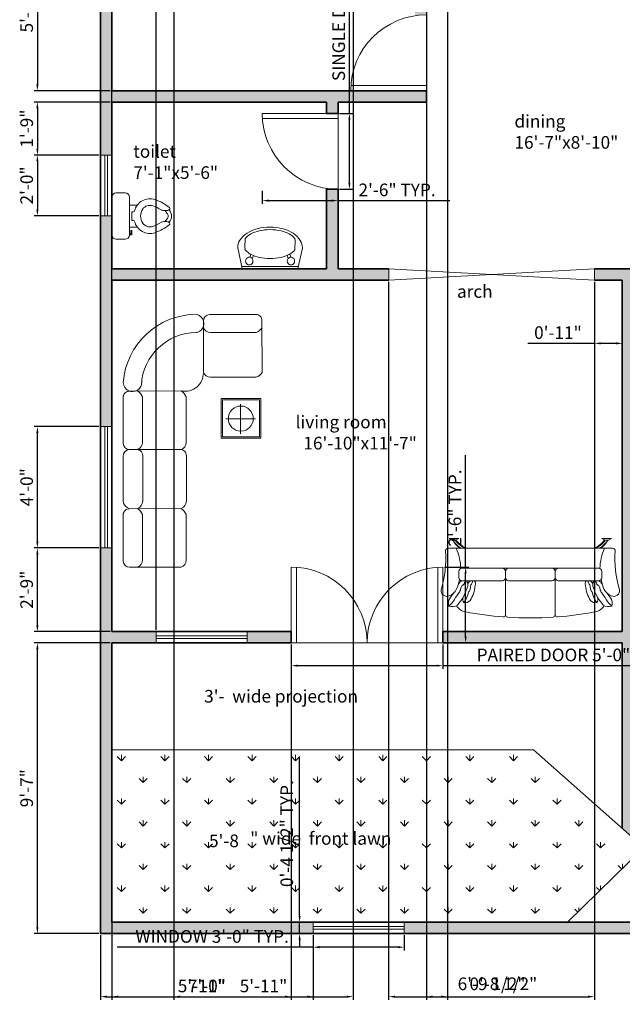
# Model space of a CAD drawing. Units: inches. Extents: x 2576 to 2974, y 2059 to 2656.
# Tile 1 of 4: x 2581 to 2819, y 2059 to 2448. Entities that reach past the tile are written whole.
import ezdxf

# ---------------------------------------------------------------- set-up
doc = ezdxf.new("R2010")
doc.units = ezdxf.units.IN
for name, color, linetype, lineweight in [('A-ANNO-DIMS', 101, 'Continuous', 18), ('A-ANNO-TEXT', 101, 'Continuous', 18), ('A-AREA-IDEN', 101, 'Continuous', 18), ('A-FLOR-FIXT', 195, 'Continuous', 18), ('A-WALL-PATT', 233, 'Continuous', 13), ('doors', 235, 'Continuous', 18), ('Furniture', 195, 'Continuous', 15), ('L-PLNT', 143, 'Continuous', 18), ('L-PLNT-PATT', 85, 'Continuous', 13), ('wall', 143, 'Continuous', 35), ('windows', 85, 'Continuous', 18)]:
    doc.layers.add(name, color=color, linetype=linetype, lineweight=lineweight)
doc.styles.get("Standard").update_dxf_attribs({"font": 'txt', "height": 5})
doc.dimstyles.new('ISO-25', dxfattribs={"dimtxt": 5, "dimasz": 2.5, "dimexe": 1.25, "dimexo": 0.625, "dimtad": 1, "dimlunit": 3, "dimtxsty": 'Standard', "dimcen": 2.5, "dimadec": 0, "dimazin": 0, "dimtfac": 1, "dimtmove": 0, "dimatfit": 3, "dimfxl": 1, "dimarcsym": 0})

# ---------------------------------------------------------------- blocks, each defined once
blk = doc.blocks.new('DOOR-SWING-30IN')
for p, q in [((0, 30), (30, 30)), ((0.07, 28), (30, 28)), ((30, 30), (30, 0))]:
    blk.add_line(p, q)
blk.add_arc((30, 30), 30, 180, 270)
blk = doc.blocks.new('DOOR-PAIR-60IN')
for p, q in [((0, 30), (0, 0)), ((2, 29.93), (2, 0)), ((58, 29.93), (58, 0)), ((60, 30), (60, 0)), ((0, 0), (30, 0)), ((60, 0), (30, 0))]:
    blk.add_line(p, q)
for centre, start, end in [((0, 0), 0, 90), ((60, 0), 90, 180)]:
    blk.add_arc(centre, 30, start, end)
blk = doc.blocks.new('WINDOW-36IN')
for p, q in [((0, 36), (0, 0)), ((4.5, 36), (0, 36)), ((1.75, 36), (1.75, 0)), ((2.75, 36), (2.75, 0)), ((4.5, 0), (4.5, 36)), ((0, 0), (4.5, 0))]:
    blk.add_line(p, q)
blk = doc.blocks.new('*D9')
at = {"layer": 'A-ANNO-DIMS', "color": 0, "lineweight": -2, "transparency": 16777216}
for p, q in [((2696.75, 2086.25), (2696.75, 2080.23)), ((2732.75, 2086.25), (2732.75, 2080.23)), ((2696.75, 2081.48), (2619.2, 2081.48)), ((2730.25, 2081.48), (2699.25, 2081.48))]:
    blk.add_line(p, q, dxfattribs=at)
at = {"layer": 'A-ANNO-DIMS', "color": 0, "transparency": 16777216}
for points in [[(2699.25, 2081.89), (2699.25, 2081.06), (2696.75, 2081.48)], [(2730.25, 2081.89), (2730.25, 2081.06), (2732.75, 2081.48)]]:
    blk.add_solid(points, dxfattribs=at)
at = {"layer": 'Defpoints', "color": 0, "transparency": 16777216}
for p in [(2696.75, 2086.88), (2732.75, 2086.88), (2696.75, 2081.48)]:
    blk.add_point(p, dxfattribs=at)
at = {"layer": 'A-ANNO-DIMS', "color": 0, "transparency": 16777216, "insert": (2656.73, 2085.08), "char_height": 5, "attachment_point": 5}
blk.add_mtext('WINDOW 3\'-0" TYP.', dxfattribs=at)
blk = doc.blocks.new('*D10')
at = {"layer": 'A-ANNO-DIMS', "color": 0, "lineweight": -2, "transparency": 16777216}
for p, q in [((2691.35, 2093.88), (2691.35, 2156.44)), ((2696.13, 2091.38), (2690.1, 2091.38)), ((2691.35, 2086.88), (2691.35, 2091.38)), ((2696.13, 2086.88), (2690.1, 2086.88)), ((2691.35, 2084.38), (2691.35, 2081.88))]:
    blk.add_line(p, q, dxfattribs=at)
at = {"layer": 'A-ANNO-DIMS', "color": 0, "transparency": 16777216}
for points in [[(2690.94, 2093.88), (2691.77, 2093.88), (2691.35, 2091.38)], [(2690.94, 2084.38), (2691.77, 2084.38), (2691.35, 2086.88)]]:
    blk.add_solid(points, dxfattribs=at)
at = {"layer": 'Defpoints', "color": 0, "transparency": 16777216}
for p in [(2691.35, 2091.38), (2696.75, 2091.38), (2696.75, 2086.88)]:
    blk.add_point(p, dxfattribs=at)
at = {"layer": 'A-ANNO-DIMS', "color": 0, "transparency": 16777216, "insert": (2686.92, 2126.41), "char_height": 5, "attachment_point": 5, "rotation": 90}
blk.add_mtext('0\'-4 1/2" TYP.', dxfattribs=at)
blk = doc.blocks.new('*D11')
at = {"layer": 'A-ANNO-DIMS', "color": 0, "lineweight": -2, "transparency": 16777216}
for p, q in [((2688.06, 2201.25), (2688.06, 2191.63)), ((2748.06, 2201.25), (2748.06, 2191.63)), ((2690.56, 2192.88), (2745.56, 2192.88)), ((2748.06, 2192.88), (2848.47, 2192.88))]:
    blk.add_line(p, q, dxfattribs=at)
at = {"layer": 'A-ANNO-DIMS', "color": 0, "transparency": 16777216}
for points in [[(2690.56, 2193.29), (2690.56, 2192.46), (2688.06, 2192.88)], [(2745.56, 2193.29), (2745.56, 2192.46), (2748.06, 2192.88)]]:
    blk.add_solid(points, dxfattribs=at)
at = {"layer": 'Defpoints', "color": 0, "transparency": 16777216}
for p in [(2688.06, 2201.88), (2748.06, 2201.88), (2748.06, 2192.88)]:
    blk.add_point(p, dxfattribs=at)
at = {"layer": 'A-ANNO-DIMS', "color": 0, "transparency": 16777216, "insert": (2799.51, 2196.48), "char_height": 5, "attachment_point": 5}
blk.add_mtext('PAIRED DOOR 5\'-0" TYP.', dxfattribs=at)
blk = doc.blocks.new('*D12')
at = {"layer": 'A-ANNO-DIMS', "color": 0, "lineweight": -2, "transparency": 16777216}
for p, q in [((2757.06, 2231.88), (2757.06, 2276.1)), ((2748.68, 2231.88), (2758.31, 2231.88)), ((2757.06, 2204.38), (2757.06, 2229.38)), ((2748.68, 2201.88), (2758.31, 2201.88))]:
    blk.add_line(p, q, dxfattribs=at)
at = {"layer": 'A-ANNO-DIMS', "color": 0, "transparency": 16777216}
for points in [[(2756.64, 2229.38), (2757.47, 2229.38), (2757.06, 2231.88)], [(2756.64, 2204.38), (2757.47, 2204.38), (2757.06, 2201.88)]]:
    blk.add_solid(points, dxfattribs=at)
at = {"layer": 'Defpoints', "color": 0, "transparency": 16777216}
for p in [(2748.06, 2231.88), (2757.06, 2231.88), (2748.06, 2201.88)]:
    blk.add_point(p, dxfattribs=at)
at = {"layer": 'A-ANNO-DIMS', "color": 0, "transparency": 16777216, "insert": (2753.46, 2255.24), "char_height": 5, "attachment_point": 5, "rotation": 90}
blk.add_mtext('2\'-6" TYP.', dxfattribs=at)
blk = doc.blocks.new('*D13')
at = {"layer": 'A-ANNO-DIMS', "color": 0, "lineweight": -2, "transparency": 16777216}
for p, q in [((2711.06, 2411.38), (2711.06, 2510.6)), ((2707.18, 2411.38), (2712.31, 2411.38)), ((2711.06, 2383.88), (2711.06, 2408.88)), ((2707.18, 2381.38), (2712.31, 2381.38))]:
    blk.add_line(p, q, dxfattribs=at)
at = {"layer": 'A-ANNO-DIMS', "color": 0, "transparency": 16777216}
for points in [[(2710.64, 2408.88), (2711.47, 2408.88), (2711.06, 2411.38)], [(2710.64, 2383.88), (2711.47, 2383.88), (2711.06, 2381.38)]]:
    blk.add_solid(points, dxfattribs=at)
at = {"layer": 'Defpoints', "color": 0, "transparency": 16777216}
for p in [(2706.56, 2411.38), (2711.06, 2411.38), (2706.56, 2381.38)]:
    blk.add_point(p, dxfattribs=at)
at = {"layer": 'A-ANNO-DIMS', "color": 0, "transparency": 16777216, "insert": (2707.46, 2462.24), "char_height": 5, "attachment_point": 5, "rotation": 90}
blk.add_mtext('SINGLE DOOR 2\'-6" TYP.', dxfattribs=at)
blk = doc.blocks.new('*D14')
at = {"layer": 'A-ANNO-DIMS', "color": 0, "lineweight": -2, "transparency": 16777216}
for p, q in [((2676.56, 2380.75), (2676.56, 2375.63)), ((2706.56, 2380.75), (2706.56, 2375.63)), ((2679.06, 2376.88), (2704.06, 2376.88)), ((2706.56, 2376.88), (2750.78, 2376.88))]:
    blk.add_line(p, q, dxfattribs=at)
at = {"layer": 'A-ANNO-DIMS', "color": 0, "transparency": 16777216}
for points in [[(2679.06, 2377.29), (2679.06, 2376.46), (2676.56, 2376.88)], [(2704.06, 2377.29), (2704.06, 2376.46), (2706.56, 2376.88)]]:
    blk.add_solid(points, dxfattribs=at)
at = {"layer": 'Defpoints', "color": 0, "transparency": 16777216}
for p in [(2676.56, 2381.38), (2706.56, 2381.38), (2706.56, 2376.88)]:
    blk.add_point(p, dxfattribs=at)
at = {"layer": 'A-ANNO-DIMS', "color": 0, "transparency": 16777216, "insert": (2729.92, 2380.48), "char_height": 5, "attachment_point": 5}
blk.add_mtext('2\'-6" TYP.', dxfattribs=at)
blk = doc.blocks.new('*D22')
at = {"layer": 'A-ANNO-DIMS', "color": 0, "lineweight": -2, "transparency": 16777216}
for p, q in [((2616.43, 2201.88), (2586.33, 2201.88)), ((2587.58, 2089.38), (2587.58, 2199.38)), ((2611.93, 2086.88), (2586.33, 2086.88))]:
    blk.add_line(p, q, dxfattribs=at)
at = {"layer": 'A-ANNO-DIMS', "color": 0, "transparency": 16777216}
for points in [[(2587.16, 2199.38), (2588, 2199.38), (2587.58, 2201.88)], [(2587.16, 2089.38), (2588, 2089.38), (2587.58, 2086.88)]]:
    blk.add_solid(points, dxfattribs=at)
at = {"layer": 'Defpoints', "color": 0, "transparency": 16777216}
for p in [(2587.58, 2201.88), (2617.06, 2201.88), (2612.56, 2086.88)]:
    blk.add_point(p, dxfattribs=at)
at = {"layer": 'A-ANNO-DIMS', "color": 0, "transparency": 16777216, "insert": (2583.98, 2144.38), "char_height": 5, "attachment_point": 5, "rotation": 90}
blk.add_mtext('9\'-7"', dxfattribs=at)
blk = doc.blocks.new('*D23')
at = {"layer": 'A-ANNO-DIMS', "color": 0, "lineweight": -2, "transparency": 16777216}
for p, q in [((2617.06, 2201.25), (2617.06, 2060.65)), ((2688.06, 2201.25), (2688.06, 2060.65)), ((2619.56, 2061.9), (2685.56, 2061.9))]:
    blk.add_line(p, q, dxfattribs=at)
at = {"layer": 'A-ANNO-DIMS', "color": 0, "transparency": 16777216}
for points in [[(2619.56, 2062.32), (2619.56, 2061.48), (2617.06, 2061.9)], [(2685.56, 2062.32), (2685.56, 2061.48), (2688.06, 2061.9)]]:
    blk.add_solid(points, dxfattribs=at)
at = {"layer": 'Defpoints', "color": 0, "transparency": 16777216}
for p in [(2617.06, 2201.88), (2688.06, 2201.88), (2688.06, 2061.9)]:
    blk.add_point(p, dxfattribs=at)
at = {"layer": 'A-ANNO-DIMS', "color": 0, "transparency": 16777216, "insert": (2652.56, 2065.5), "char_height": 5, "attachment_point": 5}
blk.add_mtext('5\'-11"', dxfattribs=at)
blk = doc.blocks.new('*D24')
at = {"layer": 'A-ANNO-DIMS', "color": 0, "lineweight": -2, "transparency": 16777216}
for p, q in [((2726.59, 2344.75), (2726.59, 2060.65)), ((2808.02, 2344.75), (2808.02, 2060.65)), ((2729.09, 2061.9), (2805.52, 2061.9))]:
    blk.add_line(p, q, dxfattribs=at)
at = {"layer": 'A-ANNO-DIMS', "color": 0, "transparency": 16777216}
for points in [[(2729.09, 2062.32), (2729.09, 2061.48), (2726.59, 2061.9)], [(2805.52, 2062.32), (2805.52, 2061.48), (2808.02, 2061.9)]]:
    blk.add_solid(points, dxfattribs=at)
at = {"layer": 'Defpoints', "color": 0, "transparency": 16777216}
for p in [(2726.59, 2345.38), (2808.02, 2345.38), (2808.02, 2061.9)]:
    blk.add_point(p, dxfattribs=at)
at = {"layer": 'A-ANNO-DIMS', "color": 0, "transparency": 16777216, "insert": (2767.31, 2066.34), "char_height": 5, "attachment_point": 5}
blk.add_mtext('6\'-9 1/2"', dxfattribs=at)
blk = doc.blocks.new('*D29')
at = {"layer": 'A-ANNO-DIMS', "color": 0, "lineweight": -2, "transparency": 16777216}
for p, q in [((2611.93, 2394.88), (2586.33, 2394.88)), ((2587.58, 2392.38), (2587.58, 2373.38)), ((2611.93, 2370.88), (2586.33, 2370.88))]:
    blk.add_line(p, q, dxfattribs=at)
at = {"layer": 'A-ANNO-DIMS', "color": 0, "transparency": 16777216}
for points in [[(2587.16, 2392.38), (2588, 2392.38), (2587.58, 2394.88)], [(2587.16, 2373.38), (2588, 2373.38), (2587.58, 2370.88)]]:
    blk.add_solid(points, dxfattribs=at)
at = {"layer": 'Defpoints', "color": 0, "transparency": 16777216}
for p in [(2612.56, 2394.88), (2587.58, 2370.88), (2612.56, 2370.88)]:
    blk.add_point(p, dxfattribs=at)
at = {"layer": 'A-ANNO-DIMS', "color": 0, "transparency": 16777216, "insert": (2583.98, 2382.88), "char_height": 5, "attachment_point": 5, "rotation": 90}
blk.add_mtext('2\'-0"', dxfattribs=at)
blk = doc.blocks.new('*D30')
at = {"layer": 'A-ANNO-DIMS', "color": 0, "lineweight": -2, "transparency": 16777216}
for p, q in [((2616.43, 2415.88), (2586.33, 2415.88)), ((2587.58, 2413.38), (2587.58, 2397.38)), ((2611.93, 2394.88), (2586.33, 2394.88))]:
    blk.add_line(p, q, dxfattribs=at)
at = {"layer": 'A-ANNO-DIMS', "color": 0, "transparency": 16777216}
for points in [[(2587.16, 2413.38), (2588, 2413.38), (2587.58, 2415.88)], [(2587.16, 2397.38), (2588, 2397.38), (2587.58, 2394.88)]]:
    blk.add_solid(points, dxfattribs=at)
at = {"layer": 'Defpoints', "color": 0, "transparency": 16777216}
for p in [(2617.06, 2415.88), (2587.58, 2394.88), (2612.56, 2394.88)]:
    blk.add_point(p, dxfattribs=at)
at = {"layer": 'A-ANNO-DIMS', "color": 0, "transparency": 16777216, "insert": (2583.98, 2405.38), "char_height": 5, "attachment_point": 5, "rotation": 90}
blk.add_mtext('1\'-9"', dxfattribs=at)
blk = doc.blocks.new('*D31')
at = {"layer": 'A-ANNO-DIMS', "color": 0, "lineweight": -2, "transparency": 16777216}
for p, q in [((2611.93, 2287.46), (2586.33, 2287.46)), ((2587.58, 2241.96), (2587.58, 2284.96)), ((2611.93, 2239.46), (2586.33, 2239.46))]:
    blk.add_line(p, q, dxfattribs=at)
at = {"layer": 'A-ANNO-DIMS', "color": 0, "transparency": 16777216}
for points in [[(2587.16, 2284.96), (2588, 2284.96), (2587.58, 2287.46)], [(2587.16, 2241.96), (2588, 2241.96), (2587.58, 2239.46)]]:
    blk.add_solid(points, dxfattribs=at)
at = {"layer": 'Defpoints', "color": 0, "transparency": 16777216}
for p in [(2587.58, 2287.46), (2612.56, 2287.46), (2612.56, 2239.46)]:
    blk.add_point(p, dxfattribs=at)
at = {"layer": 'A-ANNO-DIMS', "color": 0, "transparency": 16777216, "insert": (2583.98, 2263.46), "char_height": 5, "attachment_point": 5, "rotation": 90}
blk.add_mtext('4\'-0"', dxfattribs=at)
blk = doc.blocks.new('*D32')
at = {"layer": 'A-ANNO-DIMS', "color": 0, "lineweight": -2, "transparency": 16777216}
for p, q in [((2611.93, 2239.46), (2586.33, 2239.46)), ((2587.58, 2208.88), (2587.58, 2236.96)), ((2616.43, 2206.38), (2586.33, 2206.38))]:
    blk.add_line(p, q, dxfattribs=at)
at = {"layer": 'A-ANNO-DIMS', "color": 0, "transparency": 16777216}
for points in [[(2587.16, 2236.96), (2588, 2236.96), (2587.58, 2239.46)], [(2587.16, 2208.88), (2588, 2208.88), (2587.58, 2206.38)]]:
    blk.add_solid(points, dxfattribs=at)
at = {"layer": 'Defpoints', "color": 0, "transparency": 16777216}
for p in [(2587.58, 2239.46), (2612.56, 2239.46), (2617.06, 2206.38)]:
    blk.add_point(p, dxfattribs=at)
at = {"layer": 'A-ANNO-DIMS', "color": 0, "transparency": 16777216, "insert": (2583.98, 2222.92), "char_height": 5, "attachment_point": 5, "rotation": 90}
blk.add_mtext('2\'-9"', dxfattribs=at)
blk = doc.blocks.new('*D34')
at = {"layer": 'A-ANNO-DIMS', "color": 0, "lineweight": -2, "transparency": 16777216}
for p, q in [((2741.56, 2455.25), (2741.56, 2060.65)), ((2749.82, 2455.25), (2749.82, 2060.65)), ((2744.06, 2061.9), (2747.32, 2061.9)), ((2749.82, 2061.9), (2791.66, 2061.9))]:
    blk.add_line(p, q, dxfattribs=at)
at = {"layer": 'A-ANNO-DIMS', "color": 0, "transparency": 16777216}
for points in [[(2744.06, 2062.32), (2744.06, 2061.48), (2741.56, 2061.9)], [(2747.32, 2062.32), (2747.32, 2061.48), (2749.82, 2061.9)]]:
    blk.add_solid(points, dxfattribs=at)
at = {"layer": 'Defpoints', "color": 0, "transparency": 16777216}
for p in [(2741.56, 2455.88), (2749.82, 2455.88), (2749.82, 2061.9)]:
    blk.add_point(p, dxfattribs=at)
at = {"layer": 'A-ANNO-DIMS', "color": 0, "transparency": 16777216, "insert": (2771.99, 2066.34), "char_height": 5, "attachment_point": 5}
blk.add_mtext('0\'-8 1/2"', dxfattribs=at)
blk = doc.blocks.new('*D35')
at = {"layer": 'A-ANNO-DIMS', "color": 0, "lineweight": -2, "transparency": 16777216}
for p, q in [((2617.06, 2207), (2617.06, 2593.1)), ((2619.56, 2591.85), (2632.06, 2591.85)), ((2634.56, 2207), (2634.56, 2593.1)), ((2634.56, 2591.85), (2675.45, 2591.85))]:
    blk.add_line(p, q, dxfattribs=at)
at = {"layer": 'A-ANNO-DIMS', "color": 0, "transparency": 16777216}
for points in [[(2619.56, 2592.27), (2619.56, 2591.43), (2617.06, 2591.85)], [(2632.06, 2592.27), (2632.06, 2591.43), (2634.56, 2591.85)]]:
    blk.add_solid(points, dxfattribs=at)
at = {"layer": 'Defpoints', "color": 0, "transparency": 16777216}
for p in [(2634.56, 2591.85), (2617.06, 2206.38), (2634.56, 2206.38)]:
    blk.add_point(p, dxfattribs=at)
at = {"layer": 'A-ANNO-DIMS', "color": 0, "transparency": 16777216, "insert": (2656.25, 2596.29), "char_height": 5, "attachment_point": 5}
blk.add_mtext('1\'-5 1/2"', dxfattribs=at)
blk = doc.blocks.new('*D37')
at = {"layer": 'A-ANNO-DIMS', "color": 0, "lineweight": -2, "transparency": 16777216}
for p, q in [((2612.56, 2086.25), (2612.56, 2060.65)), ((2696.75, 2086.25), (2696.75, 2060.65)), ((2615.06, 2061.9), (2694.25, 2061.9))]:
    blk.add_line(p, q, dxfattribs=at)
at = {"layer": 'A-ANNO-DIMS', "color": 0, "transparency": 16777216}
for points in [[(2615.06, 2062.32), (2615.06, 2061.48), (2612.56, 2061.9)], [(2694.25, 2062.32), (2694.25, 2061.48), (2696.75, 2061.9)]]:
    blk.add_solid(points, dxfattribs=at)
at = {"layer": 'Defpoints', "color": 0, "transparency": 16777216}
for p in [(2612.56, 2086.88), (2696.75, 2086.88), (2696.75, 2061.9)]:
    blk.add_point(p, dxfattribs=at)
at = {"layer": 'A-ANNO-DIMS', "color": 0, "transparency": 16777216, "insert": (2654.66, 2065.5), "char_height": 5, "attachment_point": 5}
blk.add_mtext('7\'-0"', dxfattribs=at)
blk = doc.blocks.new('*D39')
at = {"layer": 'A-ANNO-DIMS', "color": 0, "lineweight": -2, "transparency": 16777216}
for p, q in [((2641.62, 2484.83), (2641.62, 2060.65)), ((2712.49, 2484.83), (2712.49, 2060.65)), ((2644.12, 2061.9), (2709.99, 2061.9))]:
    blk.add_line(p, q, dxfattribs=at)
at = {"layer": 'A-ANNO-DIMS', "color": 0, "transparency": 16777216}
for points in [[(2644.12, 2062.32), (2644.12, 2061.48), (2641.62, 2061.9)], [(2709.99, 2062.32), (2709.99, 2061.48), (2712.49, 2061.9)]]:
    blk.add_solid(points, dxfattribs=at)
at = {"layer": 'Defpoints', "color": 0, "transparency": 16777216}
for p in [(2641.62, 2485.45), (2712.49, 2485.45), (2712.49, 2061.9)]:
    blk.add_point(p, dxfattribs=at)
at = {"layer": 'A-ANNO-DIMS', "color": 0, "transparency": 16777216, "insert": (2677.06, 2065.5), "char_height": 5, "attachment_point": 5}
blk.add_mtext('5\'-11"', dxfattribs=at)
blk = doc.blocks.new('*D40')
at = {"layer": 'A-ANNO-DIMS', "color": 0, "lineweight": -2, "transparency": 16777216}
for p, q in [((2644.94, 2481.52), (2586.33, 2481.52)), ((2587.58, 2479.02), (2587.58, 2422.88)), ((2616.43, 2420.38), (2586.33, 2420.38))]:
    blk.add_line(p, q, dxfattribs=at)
at = {"layer": 'A-ANNO-DIMS', "color": 0, "transparency": 16777216}
for points in [[(2587.16, 2479.02), (2588, 2479.02), (2587.58, 2481.52)], [(2587.16, 2422.88), (2588, 2422.88), (2587.58, 2420.38)]]:
    blk.add_solid(points, dxfattribs=at)
at = {"layer": 'Defpoints', "color": 0, "transparency": 16777216}
for p in [(2645.56, 2481.52), (2587.58, 2420.38), (2617.06, 2420.38)]:
    blk.add_point(p, dxfattribs=at)
at = {"layer": 'A-ANNO-DIMS', "color": 0, "transparency": 16777216, "insert": (2583.98, 2450.95), "char_height": 5, "attachment_point": 5, "rotation": 90}
blk.add_mtext('5\'-1"', dxfattribs=at)
blk = doc.blocks.new('*D41')
at = {"layer": 'A-ANNO-DIMS', "color": 0, "lineweight": -2, "transparency": 16777216}
for p, q in [((2808.02, 2344.75), (2808.02, 2319.15)), ((2819.06, 2344.75), (2819.06, 2319.15)), ((2808.02, 2320.4), (2781.65, 2320.4)), ((2816.56, 2320.4), (2810.52, 2320.4))]:
    blk.add_line(p, q, dxfattribs=at)
at = {"layer": 'A-ANNO-DIMS', "color": 0, "transparency": 16777216}
for points in [[(2810.52, 2320.82), (2810.52, 2319.98), (2808.02, 2320.4)], [(2816.56, 2320.82), (2816.56, 2319.98), (2819.06, 2320.4)]]:
    blk.add_solid(points, dxfattribs=at)
at = {"layer": 'Defpoints', "color": 0, "transparency": 16777216}
for p in [(2808.02, 2345.38), (2819.06, 2345.38), (2808.02, 2320.4)]:
    blk.add_point(p, dxfattribs=at)
at = {"layer": 'A-ANNO-DIMS', "color": 0, "transparency": 16777216, "insert": (2793.58, 2324), "char_height": 5, "attachment_point": 5}
blk.add_mtext('0\'-11"', dxfattribs=at)

msp = doc.modelspace()

# ---------------------------------------------------------------- hatches: boundary and pattern name
at = {"layer": 'A-WALL-PATT'}
h = msp.add_hatch(color=256, dxfattribs=at)
h.dxf.hatch_style = 1
h.paths.add_polyline_path([(2726.595, 2349.876), (2706.556, 2349.876), (2706.556, 2381.376), (2702.056, 2381.376), (2702.056, 2349.876), (2617.056, 2349.876), (2617.056, 2370.876), (2612.556, 2370.876), (2612.556, 2287.457), (2617.056, 2287.457), (2617.056, 2345.376), (2726.595, 2345.376)])
h.paths.add_polyline_path([(2823.556, 2345.376), (2828.056, 2345.376), (2828.056, 2349.876), (2808.018, 2349.876), (2808.018, 2345.376), (2819.056, 2345.376), (2819.056, 2206.376), (2748.056, 2206.376), (2748.056, 2201.876), (2819.056, 2201.876), (2819.056, 2159.528), (2823.556, 2159.528)])
h.paths.add_polyline_path([(2634.556, 2206.376), (2617.056, 2206.376), (2617.056, 2239.457), (2612.556, 2239.457), (2612.556, 2086.876), (2696.755, 2086.876), (2696.755, 2091.376), (2617.056, 2091.376), (2617.056, 2201.876), (2634.556, 2201.876)])
h.paths.add_polyline_path([(2688.056, 2206.376), (2670.556, 2206.376), (2670.556, 2201.876), (2688.056, 2201.876)], flags=17)
h.paths.add_polyline_path([(2832.708, 2091.376), (2732.755, 2091.376), (2732.755, 2086.876), (2832.708, 2086.876)])
h.paths.add_polyline_path([(2823.556, 2159.528), (2819.056, 2159.528), (2819.056, 2128.522), (2823.556, 2124.554)])
h.paths.add_polyline_path([(2840.936, 2566.876), (2689.889, 2566.876), (2689.889, 2562.376), (2730.206, 2562.376), (2737.056, 2562.376), (2737.056, 2529.376), (2741.556, 2529.376), (2741.556, 2562.376), (2813.556, 2562.376), (2813.556, 2529.376), (2818.056, 2529.376), (2818.056, 2562.376), (2840.936, 2562.376)])
h.paths.add_polyline_path([(2653.889, 2566.876), (2612.556, 2566.876), (2612.556, 2509.376), (2617.056, 2509.376), (2617.056, 2562.376), (2653.889, 2562.376)])
h.paths.add_polyline_path([(2822.556, 2460.376), (2818.056, 2460.376), (2818.056, 2493.376), (2813.556, 2493.376), (2813.556, 2460.376), (2809.817, 2460.376), (2809.817, 2455.876), (2822.556, 2455.876)])
h.paths.add_polyline_path([(2912.556, 2489.593), (2908.056, 2489.593), (2908.056, 2470.164), (2908.056, 2460.376), (2852.556, 2460.376), (2852.556, 2455.876), (2908.056, 2455.876), (2908.056, 2349.876), (2858.056, 2349.876), (2858.056, 2345.376), (2908.056, 2345.376), (2908.056, 2285.493), (2912.556, 2285.493)])
h.paths.add_polyline_path([(2749.817, 2460.376), (2741.556, 2460.376), (2741.556, 2493.376), (2737.056, 2493.376), (2737.056, 2450.376), (2741.556, 2450.376), (2741.556, 2455.876), (2749.817, 2455.876)])
h.paths.add_polyline_path([(2741.556, 2420.376), (2711.556, 2420.376), (2617.056, 2420.376), (2617.056, 2473.376), (2612.556, 2473.376), (2612.556, 2394.876), (2617.056, 2394.876), (2617.056, 2415.876), (2702.056, 2415.876), (2702.056, 2411.376), (2706.556, 2411.376), (2706.556, 2415.876), (2741.556, 2415.876)])
h.paths.add_polyline_path([(2912.556, 2566.876), (2876.936, 2566.876), (2876.936, 2562.376), (2908.056, 2562.376), (2908.056, 2525.593), (2912.556, 2525.593)])
h.paths.add_polyline_path([(2741.924, 2553.087), (2815.278, 2553.087), (2815.278, 2560.74), (2741.924, 2560.74)], flags=25)
at = {"layer": 'L-PLNT-PATT'}
h = msp.add_hatch(dxfattribs=at)
h.set_pattern_fill('GRASS', color=256, scale=0.48)
h.paths.add_polyline_path([(2827.63, 2120.961), (2783.902, 2159.528), (2617.056, 2159.528), (2617.056, 2091.376), (2797.373, 2091.376)])

# ---------------------------------------------------------------- linework, layer by layer
at = {"layer": 'A-FLOR-FIXT'}
for p, q in [((2617.056, 2363.311), (2617.056, 2378.185)), ((2618.806, 2379.934), (2622.306, 2379.934)), ((2624.055, 2378.185), (2624.055, 2363.311)), ((2627.117, 2375.122), (2624.055, 2375.122)), ((2637.556, 2372.935), (2638.69, 2372.935)), ((2638.868, 2371.909), (2638.108, 2372.935)), ((2624.93, 2368.998), (2624.93, 2372.498)), ((2624.93, 2372.498), (2625.6, 2372.498)), ((2625.6, 2368.998), (2624.93, 2368.998)), ((2638.868, 2369.586), (2638.108, 2368.561)), ((2627.117, 2366.374), (2624.055, 2366.374)), ((2624.493, 2365.061), (2624.493, 2363.749)), ((2624.93, 2365.061), (2624.493, 2365.061)), ((2624.93, 2363.311), (2624.93, 2365.061)), ((2637.556, 2368.561), (2638.658, 2368.561)), ((2622.306, 2361.562), (2618.806, 2361.562)), ((2624.493, 2363.749), (2624.055, 2363.749)), ((2624.055, 2363.311), (2624.93, 2363.311)), ((2669.865, 2361.948), (2669.704, 2358.329)), ((2669.924, 2362.207), (2669.89, 2362.063)), ((2689.416, 2362.158), (2689.416, 2362.161)), ((2689.597, 2361.204), (2689.465, 2361.944)), ((2689.504, 2357.582), (2689.597, 2361.204)), ((2666.87, 2358.185), (2668.666, 2350.08)), ((2669.704, 2358.329), (2669.818, 2357.613)), ((2689.398, 2357.335), (2689.491, 2357.42)), ((2689.491, 2357.42), (2689.5, 2357.431)), ((2689.5, 2357.431), (2689.504, 2357.445)), ((2689.504, 2357.582), (2689.504, 2357.451)), ((2689.504, 2357.445), (2689.504, 2357.451)), ((2692.456, 2358.015), (2690.663, 2350.08)), ((2670.031, 2353.459), (2669.942, 2352.936)), ((2670.287, 2353.919), (2670.031, 2353.459)), ((2670.679, 2354.261), (2670.287, 2353.919)), ((2671.159, 2354.442), (2670.679, 2354.261)), ((2671.671, 2354.442), (2671.159, 2354.442)), ((2672.152, 2354.261), (2671.671, 2354.442)), ((2671.729, 2354.445), (2672.057, 2355.665)), ((2672.544, 2353.919), (2672.152, 2354.261)), ((2672.799, 2353.459), (2672.544, 2353.919)), ((2672.598, 2353.782), (2673.122, 2355.154)), ((2672.888, 2352.936), (2672.799, 2353.459)), ((2686.838, 2353.964), (2686.373, 2355.237)), ((2686.529, 2353.459), (2686.44, 2352.936)), ((2686.785, 2353.919), (2686.529, 2353.459)), ((2687.177, 2354.261), (2686.785, 2353.919)), ((2687.657, 2354.442), (2687.177, 2354.261)), ((2687.89, 2354.456), (2687.445, 2355.741)), ((2688.169, 2354.442), (2687.657, 2354.442)), ((2688.65, 2354.261), (2688.169, 2354.442)), ((2689.042, 2353.919), (2688.65, 2354.261)), ((2689.297, 2353.459), (2689.042, 2353.919)), ((2689.386, 2352.936), (2689.297, 2353.459)), ((2668.666, 2350.767), (2690.663, 2350.767)), ((2668.666, 2349.876), (2668.666, 2350.284)), ((2690.663, 2349.876), (2668.666, 2349.876)), ((2669.942, 2352.936), (2670.031, 2352.412)), ((2670.031, 2352.412), (2670.287, 2351.952)), ((2670.287, 2351.952), (2670.679, 2351.611)), ((2670.679, 2351.611), (2671.159, 2351.429)), ((2671.159, 2351.429), (2671.671, 2351.429)), ((2671.671, 2351.429), (2672.152, 2351.611)), ((2672.152, 2351.611), (2672.544, 2351.952)), ((2672.544, 2351.952), (2672.799, 2352.412)), ((2672.799, 2352.412), (2672.888, 2352.936)), ((2686.44, 2352.936), (2686.529, 2352.412)), ((2686.529, 2352.412), (2686.785, 2351.952)), ((2686.785, 2351.952), (2687.177, 2351.611)), ((2687.177, 2351.611), (2687.657, 2351.429)), ((2687.657, 2351.429), (2688.169, 2351.429)), ((2688.169, 2351.429), (2688.65, 2351.611)), ((2688.65, 2351.611), (2689.042, 2351.952)), ((2689.042, 2351.952), (2689.297, 2352.412)), ((2689.297, 2352.412), (2689.386, 2352.936)), ((2690.663, 2350.284), (2690.663, 2349.876))]:
    msp.add_line(p, q, dxfattribs=at)
for centre, radius, start, end in [((2618.806, 2378.185), 1.75, 90, 180), ((2622.306, 2378.185), 1.75, 0, 90), ((2632.148, 2371.317), 6.308, 71.81635, 166.11664), ((2627.555, 2358.718), 19.715, 51.26542, 70.55996), ((2625.6, 2372.935), 0.437, 270, 346.11664), ((2633.782, 2370.748), 5.353, 147.79727, 212.20273), ((2632.148, 2371.317), 3.683, 71.81635, 142.8917), ((2627.555, 2358.718), 17.091, 57.93751, 70.55996), ((2637.556, 2374.685), 1.75, 237.93751, 270), ((2638.69, 2374.685), 1.75, 270, 314.9399), ((2637.324, 2370.748), 3.354, 313.60282, 46.39718), ((2639.617, 2373.756), 0.437, 314.9399, 51.26542), ((2625.6, 2368.561), 0.437, 13.88336, 90), ((2637.762, 2370.748), 1.604, 313.60282, 46.39718), ((2632.148, 2370.179), 6.308, 193.88336, 288.18365), ((2632.148, 2370.179), 3.683, 217.1083, 288.18365), ((2627.555, 2382.778), 17.091, 289.44004, 302.06249), ((2627.555, 2382.778), 19.715, 289.44004, 308.66501), ((2637.556, 2366.811), 1.75, 90, 122.06249), ((2638.658, 2366.811), 1.75, 44.16247, 90), ((2639.599, 2367.725), 0.437, 308.66501, 44.16247), ((2678.23, 2351.974), 14.268, 104.84096, 122.14001), ((2678.218, 2352.099), 13.138, 102.69985, 117.86942), ((2679.708, 2345.663), 20.748, 90.03161, 104.32228), ((2679.748, 2344.539), 20.85, 90.22979, 102.23443), ((2679.581, 2344.539), 20.85, 77.76557, 89.77021), ((2679.51, 2345.663), 20.749, 75.19563, 89.4863), ((2681.111, 2352.099), 13.138, 62.13058, 77.30015), ((2681.042, 2351.959), 14.271, 57.38302, 74.68206), ((2618.806, 2363.311), 1.75, 180, 270), ((2622.306, 2363.311), 1.75, 270, 0), ((2672.028, 2358.327), 5.159, 146.40841, 180.37125), ((2675.82, 2355.905), 9.658, 122.44128, 146.88872), ((2675.778, 2356.818), 7.825, 118.22812, 139.1983), ((2683.551, 2356.818), 7.825, 40.89638, 61.77231), ((2683.486, 2355.869), 9.661, 32.64614, 57.09358), ((2687.3, 2358.259), 5.16, 359.17847, 33.14131), ((2672.045, 2358.271), 5.176, 179.7541, 180.94709), ((2675.78, 2362.519), 7.829, 219.32993, 241.76567), ((2683.55, 2362.517), 7.827, 298.23024, 319.68215), ((2687.284, 2358.202), 5.176, 357.92664, 359.81125), ((2678.218, 2367.236), 13.138, 242.13058, 257.30015), ((2679.748, 2374.795), 20.85, 257.76557, 269.77021), ((2679.581, 2374.795), 20.85, 270.22979, 282.23443), ((2681.111, 2367.236), 13.138, 282.69985, 297.86942)]:
    msp.add_arc(centre, radius, start, end, dxfattribs=at)
at = {"layer": 'doors'}
for p, q in [((2767.306, 2347.626), (2726.595, 2349.876)), ((2726.595, 2349.876), (2726.595, 2345.376)), ((2767.306, 2347.626), (2808.018, 2349.876)), ((2808.018, 2349.876), (2808.018, 2345.376)), ((2726.595, 2345.376), (2767.306, 2347.626)), ((2808.018, 2345.376), (2767.306, 2347.626))]:
    msp.add_line(p, q, dxfattribs=at)
at = {"layer": 'Furniture'}
for p, q in [((2655.651, 2331.86), (2674.019, 2331.86)), ((2653.329, 2308.965), (2653.329, 2329.328)), ((2653.329, 2326.658), (2653.329, 2326.731)), ((2676.553, 2308.86), (2676.447, 2329.328)), ((2650.792, 2324.69), (2650.545, 2324.69)), ((2674.125, 2324.654), (2656.074, 2324.654)), ((2674.125, 2306.961), (2656.074, 2306.961)), ((2621.528, 2280.725), (2621.528, 2299.092)), ((2624.061, 2301.52), (2644.529, 2301.626)), ((2629.143, 2299.198), (2629.143, 2281.147)), ((2646.428, 2299.198), (2646.428, 2281.147)), ((2660.309, 2298.583, 9.783), (2660.309, 2282.89, 9.783)), ((2676.002, 2298.583, 9.783), (2660.309, 2298.583, 9.783)), ((2676.002, 2282.89, 9.783), (2676.002, 2298.583, 9.783)), ((2660.88, 2298.012, 9.783), (2660.88, 2283.46, 9.783)), ((2675.432, 2298.012, 9.783), (2660.88, 2298.012, 9.783)), ((2668.02, 2296.404, 9.783), (2668.02, 2284.648, 9.783)), ((2675.432, 2283.46, 9.783), (2675.432, 2298.012, 9.783)), ((2662.139, 2290.589, 9.783), (2673.839, 2290.589, 9.783)), ((2660.88, 2283.46, 9.783), (2675.432, 2283.46, 9.783)), ((2660.309, 2282.89, 9.783), (2676.002, 2282.89, 9.783)), ((2621.528, 2257.822), (2621.528, 2275.662)), ((2623.85, 2278.407), (2644.107, 2278.407)), ((2644.424, 2278.402), (2624.061, 2278.402)), ((2629.248, 2275.979), (2629.248, 2262.467)), ((2646.534, 2275.979), (2646.534, 2262.467)), ((2629.248, 2262.467), (2629.248, 2257.928)), ((2646.534, 2262.467), (2646.534, 2257.928)), ((2621.528, 2234.176), (2621.528, 2252.544)), ((2624.061, 2254.972), (2644.529, 2255.077)), ((2629.143, 2252.65), (2629.143, 2234.599)), ((2646.428, 2252.65), (2646.428, 2234.599)), ((2750.535, 2243.244), (2754.374, 2243.244)), ((2814.777, 2243.244), (2810.937, 2243.244)), ((2815.117, 2239.307), (2750.195, 2239.307)), ((2644.424, 2231.854), (2624.061, 2231.854)), ((2754.364, 2227.682), (2754.364, 2230.252)), ((2810.219, 2231.433), (2755.092, 2231.433)), ((2772.813, 2227.682), (2772.813, 2230.252)), ((2792.498, 2227.682), (2792.498, 2230.252)), ((2810.948, 2227.682), (2810.948, 2230.252)), ((2771.632, 2226.501), (2755.545, 2226.501)), ((2772.813, 2212.943), (2772.813, 2227.682)), ((2791.317, 2226.501), (2773.994, 2226.501)), ((2792.498, 2212.943), (2792.498, 2227.682)), ((2809.767, 2226.501), (2793.679, 2226.501)), ((2750.976, 2219.77), (2752.201, 2221.494)), ((2814.335, 2219.77), (2813.11, 2221.494))]:
    msp.add_line(p, q, dxfattribs=at)
msp.add_circle((2668.083, 2290.651, 9.783), 4.94, dxfattribs=at)
for centre, radius, start, end in [((2650.545, 2302.84), 29.053, 90.05172, 176.01296), ((2649.717, 2328.256), 3.725, 286.76651, 77.57392), ((2655.871, 2329.328), 2.542, 94.95025, 180), ((2674.019, 2329.43), 2.43, 357.59118, 90), ((2656.074, 2327.535), 2.881, 197.71123, 270), ((2671.815, 2330.108), 5.923, 292.94977, 323.1162), ((2650.545, 2302.84), 21.849, 90, 177.08406), ((2645.996, 2308.699), 7.281, 259.39938, 0), ((2656.074, 2309.842), 2.881, 197.71123, 270), ((2671.815, 2312.414), 5.923, 292.94977, 323.1162), ((2625.24, 2305.003), 3.681, 181.98787, 1.98787), ((2623.958, 2299.092), 2.43, 87.59118, 180), ((2623.689, 2296.888), 5.923, 22.94977, 53.1162), ((2640.974, 2296.888), 5.923, 22.94977, 53.1162), ((2624.061, 2280.944), 2.542, 184.95025, 270), ((2626.262, 2281.147), 2.881, 295.92568, 0), ((2643.547, 2281.147), 2.881, 287.71123, 0), ((2624.312, 2275.662), 2.783, 99.55584, 180), ((2626.822, 2275.98), 2.427, 359.97104, 73.24226), ((2644.107, 2275.98), 2.427, 359.97104, 90), ((2625.065, 2258.414), 3.586, 189.50631, 253.73201), ((2626.22, 2257.928), 3.028, 289.75888, 0), ((2643.505, 2257.928), 3.028, 289.75888, 0), ((2623.958, 2252.544), 2.43, 87.59118, 180), ((2623.689, 2250.34), 5.923, 22.94977, 53.1162), ((2640.974, 2250.34), 5.923, 22.94977, 53.1162), ((2752.455, 2245.511), 2.971, 229.74247, 310.25753), ((2762.524, 2248.826), 12.311, 210.42503, 230.63948), ((2760.49, 2247.455), 9.801, 209.84959, 235.62722), ((2760.279, 2247.522), 9.613, 211.21622, 237.77703), ((2761.376, 2248.968), 10.625, 217.88984, 241.58), ((2762.262, 2249.398), 11.427, 216.47208, 242.0167), ((2763.278, 2250.366), 12.672, 217.54413, 240.76997), ((2802.034, 2250.366), 12.672, 299.23003, 322.45587), ((2803.05, 2249.398), 11.427, 297.9833, 323.52792), ((2803.936, 2248.968), 10.625, 298.42, 322.11016), ((2805.033, 2247.522), 9.613, 302.22297, 328.78378), ((2804.821, 2247.455), 9.801, 304.37278, 330.15041), ((2802.788, 2248.826), 12.311, 309.36052, 329.57497), ((2812.857, 2245.511), 2.971, 229.74247, 310.25753), ((2709.687, 2234.942), 39.513, 342.32045, 5.03105), ((2750.195, 2238.126), 1.181, 90, 166.21722), ((2735.374, 2231.04), 19.723, 0.88271, 24.78203), ((2829.938, 2231.04), 19.723, 155.21797, 179.11729), ((2815.117, 2238.126), 1.181, 13.78278, 90), ((2855.624, 2234.942), 39.513, 174.96895, 197.67955), ((2624.061, 2234.396), 2.542, 184.95025, 270), ((2626.262, 2234.599), 2.881, 295.92568, 0), ((2643.547, 2234.599), 2.881, 287.71123, 0), ((2755.545, 2230.252), 1.181, 90, 180), ((2771.632, 2230.252), 1.181, 0, 90), ((2773.994, 2230.252), 1.181, 90, 180), ((2791.317, 2230.252), 1.181, 0, 90), ((2793.679, 2230.252), 1.181, 90, 180), ((2809.767, 2230.252), 1.181, 0, 90), ((2735.374, 2231.04), 19.723, 335.85537, 347.88917), ((2757.389, 2223.313), 3.631, 118.61875, 152.1269), ((2755.545, 2227.682), 1.181, 180, 270), ((2755.355, 2224.861), 2.6, 332.01824, 39.07485), ((2760.718, 2224.253), 2.905, 129.27969, 162.78784), ((2758.889, 2225.169), 2.08, 342.67918, 39.78078), ((2771.632, 2227.682), 1.181, 270, 0), ((2773.994, 2227.682), 1.181, 180, 270), ((2791.317, 2227.682), 1.181, 270, 0), ((2793.679, 2227.682), 1.181, 180, 270), ((2806.422, 2225.169), 2.08, 140.21922, 197.32082), ((2804.594, 2224.253), 2.905, 17.21216, 50.72031), ((2809.957, 2224.861), 2.6, 140.92515, 207.98176), ((2807.923, 2223.313), 3.631, 27.8731, 61.38125), ((2809.767, 2227.682), 1.181, 270, 0), ((2829.938, 2231.04), 19.723, 192.11083, 204.14463), ((2749.633, 2222.61), 2.323, 171.77911, 294.62774), ((2748.542, 2225.592), 5.494, 292.01287, 331.52204), ((2816.77, 2225.592), 5.494, 208.47796, 247.98713), ((2815.679, 2222.61), 2.323, 245.37226, 8.22089), ((2753.883, 2217.595), 3.631, 143.19121, 198.3312), ((2751.734, 2219.778), 3.569, 248.68819, 304.92938), ((2758.808, 2219.239), 2.905, 170.55851, 208.99214), ((2756.795, 2220.637), 2.855, 259.34913, 315.59032), ((2808.517, 2220.637), 2.855, 224.40968, 280.65087), ((2806.504, 2219.239), 2.905, 331.00786, 9.44149), ((2813.578, 2219.778), 3.569, 235.07062, 291.31181), ((2811.428, 2217.595), 3.631, 341.6688, 36.80879), ((2758.253, 2219.784), 5.797, 213.08856, 258.17772), ((2782.656, 2351.544), 139.796, 259.45221, 265.61436), ((2772.026, 2212.943), 0.787, 265.61436, 0), ((2773.826, 2213.041), 1.017, 185.54939, 260.22613), ((2791.486, 2213.041), 1.017, 279.77387, 354.45061), ((2793.286, 2212.943), 0.787, 180, 274.38564), ((2782.656, 2351.544), 139.796, 274.38564, 280.54779), ((2807.059, 2219.784), 5.797, 281.82228, 326.91144), ((2782.656, 2351.544), 139.796, 266.30772, 273.69228)]:
    msp.add_arc(centre, radius, start, end, dxfattribs=at)
for points, knots in [([(2750.437, 2216.453), (2750.809, 2216.776), (2751.463, 2217.343), (2752.697, 2218.952), (2753.571, 2220.876), (2755.164, 2222.571), (2755.084, 2224.371), (2756.533, 2225.021), (2756.672, 2225.995), (2756.788, 2226.41), (2756.815, 2226.501)], [0, 0, 0, 0, 37.5062875, 65.7822589, 153.6196579, 198.4652852, 236.4958826, 274.8371613, 300.2428421, 307.4283796, 307.4283796, 307.4283796, 307.4283796]), ([(2756.267, 2217.831), (2756.512, 2218.14), (2756.943, 2218.682), (2757.674, 2220.13), (2758.077, 2221.772), (2759.078, 2223.341), (2758.749, 2224.744), (2759.792, 2225.469), (2759.76, 2226.195), (2759.778, 2226.483), (2759.779, 2226.501)], [0, 0, 0, 0, 37.5062875, 65.7822589, 153.6196579, 198.4652852, 236.4958826, 274.8371613, 300.2428421, 301.9269714, 301.9269714, 301.9269714, 301.9269714]), ([(2758.835, 2218.639), (2759.335, 2219.531), (2760.371, 2221.377), (2760.703, 2223.469), (2760.875, 2224.55)], [0, 0, 0, 0, 3.0435999, 6.2979445, 6.2979445, 6.2979445, 6.2979445]), ([(2806.477, 2218.639), (2805.976, 2219.531), (2804.94, 2221.377), (2804.608, 2223.469), (2804.437, 2224.55)], [0, 0, 0, 0, 3.0435999, 6.2979445, 6.2979445, 6.2979445, 6.2979445]), ([(2809.045, 2217.831), (2808.799, 2218.14), (2808.369, 2218.682), (2807.637, 2220.13), (2807.235, 2221.772), (2806.234, 2223.341), (2806.563, 2224.744), (2805.52, 2225.469), (2805.552, 2226.195), (2805.534, 2226.483), (2805.532, 2226.501)], [0, 0, 0, 0, 37.5062875, 65.7822589, 153.6196579, 198.4652852, 236.4958826, 274.8371613, 300.2428421, 301.9269714, 301.9269714, 301.9269714, 301.9269714]), ([(2814.875, 2216.453), (2814.502, 2216.776), (2813.848, 2217.343), (2812.615, 2218.952), (2811.74, 2220.876), (2810.148, 2222.571), (2810.228, 2224.371), (2808.779, 2225.021), (2808.639, 2225.995), (2808.524, 2226.41), (2808.497, 2226.501)], [0, 0, 0, 0, 37.5062875, 65.7822589, 153.6196579, 198.4652852, 236.4958826, 274.8371613, 300.2428421, 307.4283796, 307.4283796, 307.4283796, 307.4283796]), ([(2753.778, 2216.851), (2754.599, 2217.832), (2756.298, 2219.86), (2757.19, 2222.353), (2757.651, 2223.641)], [0, 0, 0, 0, 3.8044998, 7.8724306, 7.8724306, 7.8724306, 7.8724306]), ([(2811.534, 2216.851), (2810.713, 2217.832), (2809.013, 2219.86), (2808.122, 2222.353), (2807.661, 2223.641)], [0, 0, 0, 0, 3.8044998, 7.8724306, 7.8724306, 7.8724306, 7.8724306])]:
    msp.add_open_spline(points, degree=3, knots=knots, dxfattribs=at)
at = {"layer": 'L-PLNT'}
for p, q in [((2617.056, 2159.528), (2783.902, 2159.528)), ((2783.902, 2159.528), (2827.63, 2120.961)), ((2827.63, 2120.961), (2797.373, 2091.376))]:
    msp.add_line(p, q, dxfattribs=at)
at = {"layer": 'wall'}
for p, q in [((2612.556, 2086.876), (2612.556, 2566.876)), ((2617.056, 2420.376), (2617.056, 2562.376)), ((2617.056, 2420.376), (2737.056, 2420.376)), ((2737.056, 2420.376), (2741.556, 2420.376)), ((2741.556, 2415.876), (2741.556, 2420.376)), ((2617.056, 2415.876), (2702.056, 2415.876)), ((2617.056, 2349.876), (2617.056, 2415.876)), ((2702.056, 2411.376), (2702.056, 2415.876)), ((2706.556, 2415.876), (2741.556, 2415.876)), ((2706.556, 2411.376), (2706.556, 2415.876)), ((2702.056, 2411.376), (2706.556, 2411.376)), ((2702.056, 2349.876), (2702.056, 2381.376)), ((2702.056, 2381.376), (2706.556, 2381.376)), ((2706.556, 2349.876), (2706.556, 2381.376)), ((2617.056, 2349.876), (2702.056, 2349.876)), ((2706.556, 2349.876), (2726.595, 2349.876)), ((2808.018, 2349.876), (2828.056, 2349.876)), ((2617.056, 2345.376), (2726.595, 2345.376)), ((2617.056, 2206.376), (2617.056, 2345.376)), ((2808.018, 2345.376), (2819.056, 2345.376)), ((2819.056, 2206.376), (2819.056, 2345.376)), ((2617.056, 2206.376), (2688.056, 2206.376)), ((2688.056, 2206.376), (2688.056, 2201.876)), ((2748.056, 2206.376), (2748.056, 2201.876)), ((2748.056, 2206.376), (2819.056, 2206.376)), ((2617.056, 2091.376), (2617.056, 2201.876)), ((2617.056, 2201.876), (2688.056, 2201.876)), ((2748.056, 2201.876), (2819.056, 2201.876)), ((2819.056, 2128.522), (2819.056, 2201.876)), ((2832.708, 2091.376), (2617.056, 2091.376)), ((2832.708, 2086.876), (2612.556, 2086.876))]:
    msp.add_line(p, q, dxfattribs=at)
at = {"layer": 'windows'}
for p, q in [((2612.556, 2394.876), (2612.556, 2370.876)), ((2617.056, 2394.876), (2612.556, 2394.876)), ((2614.306, 2394.876), (2614.306, 2370.876)), ((2615.306, 2394.876), (2615.306, 2370.876)), ((2617.056, 2370.876), (2617.056, 2394.876)), ((2612.556, 2370.876), (2617.056, 2370.876)), ((2612.556, 2287.457), (2612.556, 2239.457)), ((2617.056, 2287.457), (2612.556, 2287.457)), ((2614.306, 2287.457), (2614.306, 2239.457)), ((2615.306, 2287.457), (2615.306, 2239.457)), ((2617.056, 2239.457), (2617.056, 2287.457)), ((2612.556, 2239.457), (2617.056, 2239.457))]:
    msp.add_line(p, q, dxfattribs=at)

# ---------------------------------------------------------------- block references
at = {"layer": 'doors', "extrusion": (0, 0, -1), "zscale": -1, "rotation": 180}
msp.add_blockref('DOOR-SWING-30IN', (-2711.556, 2450.376), dxfattribs=at)
at = {"layer": 'doors'}
for name, p in [('DOOR-SWING-30IN', (2676.556, 2381.376)), ('DOOR-PAIR-60IN', (2688.056, 2201.876))]:
    msp.add_blockref(name, p, dxfattribs=at)
at = {"layer": 'windows'}
for p, rotation in [((2670.556, 2201.876), 89.99999999999731), ((2732.755, 2086.876), 89.99999999999767)]:
    msp.add_blockref('WINDOW-36IN', p, dxfattribs=dict(at, rotation=rotation))

# ---------------------------------------------------------------- texts
at = {"layer": 'A-ANNO-TEXT'}
for s, p in [('arch', (2753.616, 2338.423)), ("3'-  wide projection", (2653.573, 2178.269)), ('" wide  front lawn', (2671.806, 2122.019)), ("5'-8", (2655.492, 2121.061))]:
    msp.add_text(s, height=5, dxfattribs=at).set_placement(p)
at = {"layer": 'A-AREA-IDEN'}
for s, p in [('dining ', (2776.375, 2405.784)), ('16\'-7"x8\'-10"', (2776.375, 2397.415)), ('toilet', (2625.551, 2393.828)), ('7\'-1"x5\'-6"', (2625.551, 2385.46)), ('living room', (2689.783, 2286.78)), ('  16\'-10"x11\'-7"', (2689.783, 2278.412))]:
    msp.add_text(s, height=5, dxfattribs=at).set_placement(p)

# ---------------------------------------------------------------- dimensions: what is measured, and where the dimension line sits
at = {"layer": 'A-ANNO-DIMS'}
for base, p1, p2, picture, middle in [((2634.556, 2591.851), (2617.056, 2206.376), (2634.556, 2206.376), '*D35', (2656.253, 2596.285)), ((2712.489, 2061.901), (2641.623, 2485.455), (2712.489, 2485.455), '*D39', (2677.056, 2065.502)), ((2749.817, 2061.901), (2741.556, 2455.876), (2749.817, 2455.876), '*D34', (2771.989, 2066.335)), ((2808.018, 2061.901), (2726.595, 2345.376), (2808.018, 2345.376), '*D24', (2767.306, 2066.335)), ((2688.056, 2061.901), (2617.056, 2201.876), (2688.056, 2201.876), '*D23', (2652.556, 2065.502)), ((2696.755, 2061.901), (2612.556, 2086.876), (2696.755, 2086.876), '*D37', (2654.655, 2065.502))]:
    dim = msp.add_linear_dim(base=base, p1=p1, p2=p2, dimstyle='ISO-25', override={"dimdec": 1, "dimlfac": 1, "dimrnd": 0, "dimzin": 1, "dimdsep": 46, "dimlunit": 4, "dimfrac": 2}, dxfattribs=at)
    dim.commit()
    dim.dimension.update_dxf_attribs({"geometry": picture, "text_midpoint": middle})
for base, p1, p2, angle, text, picture, middle in [((2711.056, 2411.376), (2706.556, 2381.376), (2706.556, 2411.376), 90, 'SINGLE DOOR <> TYP.', '*D13', (2707.455, 2462.239)), ((2757.056, 2231.876), (2748.056, 2201.876), (2748.056, 2231.876), 90, '<> TYP.', '*D12', (2753.455, 2255.239)), ((2691.355, 2091.376), (2696.755, 2086.876), (2696.755, 2091.376), 90, '<> TYP.', '*D10', (2686.92, 2126.406)), ((2696.755, 2081.476), (2732.755, 2086.876), (2696.755, 2086.876), 180, 'WINDOW <> TYP.', '*D9', (2656.725, 2085.077))]:
    dim = msp.add_linear_dim(base=base, p1=p1, p2=p2, angle=angle, text=text, dimstyle='ISO-25', override={"dimdec": 1, "dimlfac": 1, "dimrnd": 0, "dimzin": 1, "dimdsep": 46, "dimlunit": 4, "dimfrac": 2}, dxfattribs=at)
    dim.commit()
    dim.dimension.update_dxf_attribs({"geometry": picture, "text_midpoint": middle})
for base, p1, p2, angle, picture, middle in [((2587.581, 2420.376), (2645.56, 2481.518), (2617.056, 2420.376), 90, '*D40', (2583.98, 2450.947)), ((2587.581, 2394.876), (2617.056, 2415.876), (2612.556, 2394.876), 90, '*D30', (2583.98, 2405.376)), ((2587.581, 2370.876), (2612.556, 2394.876), (2612.556, 2370.876), 90, '*D29', (2583.98, 2382.876)), ((2808.018, 2320.401), (2819.056, 2345.376), (2808.018, 2345.376), 180, '*D41', (2793.583, 2324.002)), ((2587.581, 2287.457), (2612.556, 2239.457), (2612.556, 2287.457), 90, '*D31', (2583.98, 2263.457)), ((2587.581, 2239.457), (2617.056, 2206.376), (2612.556, 2239.457), 90, '*D32', (2583.98, 2222.916)), ((2587.581, 2201.876), (2612.556, 2086.876), (2617.056, 2201.876), 90, '*D22', (2583.98, 2144.376))]:
    dim = msp.add_linear_dim(base=base, p1=p1, p2=p2, angle=angle, dimstyle='ISO-25', override={"dimdec": 1, "dimlfac": 1, "dimrnd": 0, "dimzin": 1, "dimdsep": 46, "dimlunit": 4, "dimfrac": 2}, dxfattribs=at)
    dim.commit()
    dim.dimension.update_dxf_attribs({"geometry": picture, "text_midpoint": middle})
for base, p1, p2, text, picture, middle in [((2706.556, 2376.876), (2676.556, 2381.376), (2706.556, 2381.376), '<> TYP.', '*D14', (2729.919, 2380.477)), ((2748.056, 2192.876), (2688.056, 2201.876), (2748.056, 2201.876), 'PAIRED DOOR <> TYP.', '*D11', (2799.515, 2196.477))]:
    dim = msp.add_linear_dim(base=base, p1=p1, p2=p2, text=text, dimstyle='ISO-25', override={"dimdec": 1, "dimlfac": 1, "dimrnd": 0, "dimzin": 1, "dimdsep": 46, "dimlunit": 4, "dimfrac": 2}, dxfattribs=at)
    dim.commit()
    dim.dimension.update_dxf_attribs({"geometry": picture, "text_midpoint": middle})

doc.saveas('drawing.dxf')
